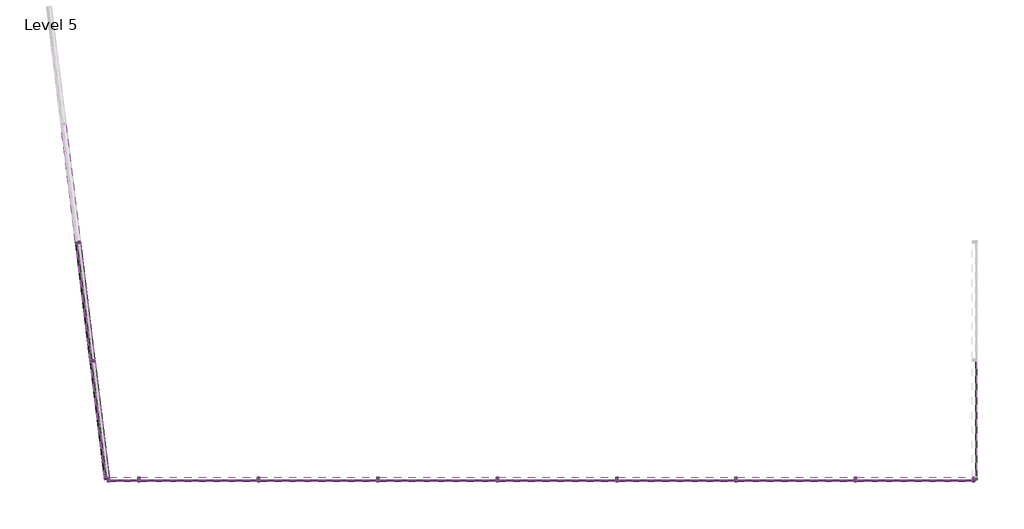
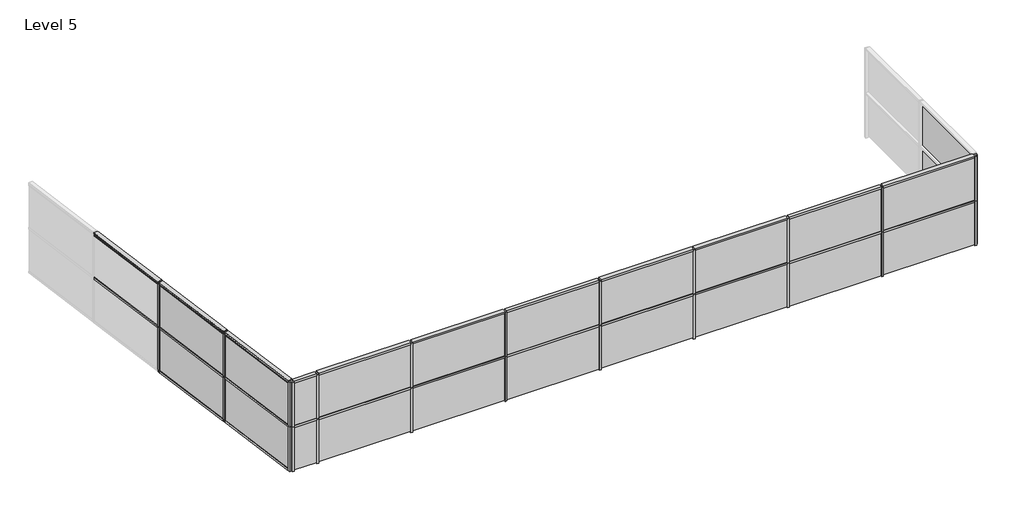
# One storey, part 1 of 2: 62 members, 26 plates.
"""IFC4 building model written with IfcOpenShell, lengths in millimetres."""

from ifc_helpers import new_model, si_unit, origin, place, context, project, spatial, transform, mapped, element, save
from components import member_71c27fd2, member_daa7a266, member_82905deb, member_19d0a4ec, member_8cef0660, member_db480205, member_4491d118, member_0c11e56c, system_panel_glazed_37f15d2e, system_panel_glazed_3620f98e, system_panel_glazed_e46d4b42, system_panel_glazed_2a6c68b7, system_panel_glazed_9d0e0944

model = new_model("IFC4")

# Units and contexts
model_context = context("Model", 3, world=origin())
ifc_project = project(units=[si_unit("LENGTHUNIT", "METRE", prefix="MILLI")], contexts=[model_context])

# Site, building, storey
site = spatial("IfcSite", under=ifc_project)
building = spatial("IfcBuilding", under=site)
storey = spatial("IfcBuildingStorey", under=building, Name="Level 5", Elevation=12192.0)

# Members
placement = place(None, origin())
member_shape = member_71c27fd2(model_context)
element("IfcMember", 1, ObjectType="Rectangular Mullion : 2.5\" x 5\" rectangular", at=placement, inside=storey, context=model_context, shape_type="MappedRepresentation", body=[
    mapped(member_shape, transform((-8620.3262186, -3985.3690403, 12192.0), x_axis=(0.0, 0.0, -1.0), y_axis=(-0.9925461516413222, -0.12186934340514607, 0.0), z_axis=(-0.12186934340514607, 0.9925461516413222, 0.0))),
])
member_2_shape = member_daa7a266(model_context)
element("IfcMember", 2, ObjectType="Rectangular Mullion : 2.5\" x 5\" rectangular", at=placement, inside=storey, context=model_context, shape_type="MappedRepresentation", body=[
    mapped(member_2_shape, transform((-8260.4765148, -6916.1096898, 15240.0), x_axis=(0.0, 0.0, 1.0), y_axis=(-0.9925461516413222, -0.12186934340514587, 0.0), z_axis=(0.12186934340514587, -0.9925461516413222, 0.0))),
])
member_3_shape = member_82905deb(model_context)
element("IfcMember", 3, ObjectType="Rectangular Mullion : 2.5\" x 5\" rectangular", at=placement, inside=storey, context=model_context, shape_type="MappedRepresentation", body=[
    mapped(member_3_shape, transform((-8624.1955702, -3953.8557, 15240.0), x_axis=(-0.1218693434051459, 0.9925461516413222, 0.0), y_axis=(-0.9925461516413222, -0.1218693434051459, 0.0), z_axis=(0.0, 0.0, 1.0))),
])
element("IfcMember", 4, ObjectType="Rectangular Mullion : 2.5\" x 5\" rectangular", at=placement, inside=storey, context=model_context, shape_type="MappedRepresentation", body=[
    mapped(member_3_shape, transform((-8995.6533289, -928.5750297, 15240.0), x_axis=(-0.1218693434051459, 0.9925461516413222, 0.0), y_axis=(-0.9925461516413222, -0.1218693434051459, 0.0), z_axis=(0.0, 0.0, 1.0))),
])
member_4_shape = member_19d0a4ec(model_context)
element("IfcMember", 5, ObjectType="Rectangular Mullion : 2.5\" x 5\" rectangular", at=placement, inside=storey, context=model_context, shape_type="MappedRepresentation", body=[
    mapped(member_4_shape, transform((13839.0156363, -6979.1363705, 13716.0), x_axis=(0.0, 0.0, 1.0), y_axis=(0.0, -1.0, 0.0), z_axis=(1.0, 0.0, 0.0))),
])
element("IfcMember", 6, ObjectType="Rectangular Mullion : 2.5\" x 5\" rectangular", at=placement, inside=storey, context=model_context, shape_type="MappedRepresentation", body=[
    mapped(member_4_shape, transform((13839.0156363, -6979.1363705, 15240.0), x_axis=(0.0, 0.0, 1.0), y_axis=(0.0, -1.0, 0.0), z_axis=(1.0, 0.0, 0.0))),
])
element("IfcMember", 7, ObjectType="Rectangular Mullion : 2.5\" x 5\" rectangular", at=placement, inside=storey, context=model_context, shape_type="MappedRepresentation", body=[
    mapped(member_4_shape, transform((-8260.4765148, -6916.1096898, 13716.0), x_axis=(0.0, 0.0, 1.0), y_axis=(-0.9925461516413222, -0.12186934340514591, 0.0), z_axis=(0.12186934340514591, -0.9925461516413222, 0.0))),
])
element("IfcMember", 8, ObjectType="Rectangular Mullion : 2.5\" x 5\" rectangular", at=placement, inside=storey, context=model_context, shape_type="MappedRepresentation", body=[
    mapped(member_4_shape, transform((-8260.4765148, -6916.1096898, 15240.0), x_axis=(0.0, 0.0, 1.0), y_axis=(-0.9925461516413223, -0.12186934340514578, 0.0), z_axis=(0.12186934340514578, -0.9925461516413223, 0.0))),
])
element("IfcMember", 9, ObjectType="Rectangular Mullion : 2.5\" x 5\" rectangular", at=placement, inside=storey, context=model_context, shape_type="MappedRepresentation", body=[
    mapped(member_4_shape, transform((-8260.4765148, -6916.1096898, 13716.0), x_axis=(0.0, 0.0, 1.0), y_axis=(-0.9925461516413223, -0.1218693434051456, 0.0), z_axis=(0.12186934340514559, -0.9925461516413222, 0.0))),
])
member_5_shape = member_8cef0660(model_context)
element("IfcMember", 10, ObjectType="Rectangular Mullion : 2.5\" x 5\" rectangular", at=placement, inside=storey, context=model_context, shape_type="MappedRepresentation", body=[
    mapped(member_5_shape, transform((10822.765636, -6979.1363705, 13716.0), x_axis=(0.0, 0.0, 1.0), y_axis=(0.0, -1.0, 0.0), z_axis=(1.0, 0.0, 0.0))),
])
element("IfcMember", 11, ObjectType="Rectangular Mullion : 2.5\" x 5\" rectangular", at=placement, inside=storey, context=model_context, shape_type="MappedRepresentation", body=[
    mapped(member_5_shape, transform((7774.765636, -6979.1363705, 13716.0), x_axis=(0.0, 0.0, 1.0), y_axis=(0.0, -1.0, 0.0), z_axis=(1.0, 0.0, 0.0))),
])
element("IfcMember", 12, ObjectType="Rectangular Mullion : 2.5\" x 5\" rectangular", at=placement, inside=storey, context=model_context, shape_type="MappedRepresentation", body=[
    mapped(member_5_shape, transform((4726.765636, -6979.1363705, 13716.0), x_axis=(0.0, 0.0, 1.0), y_axis=(0.0, -1.0, 0.0), z_axis=(1.0, 0.0, 0.0))),
])
element("IfcMember", 13, ObjectType="Rectangular Mullion : 2.5\" x 5\" rectangular", at=placement, inside=storey, context=model_context, shape_type="MappedRepresentation", body=[
    mapped(member_5_shape, transform((1678.765636, -6979.1363705, 13716.0), x_axis=(0.0, 0.0, 1.0), y_axis=(0.0, -1.0, 0.0), z_axis=(1.0, 0.0, 0.0))),
])
element("IfcMember", 14, ObjectType="Rectangular Mullion : 2.5\" x 5\" rectangular", at=placement, inside=storey, context=model_context, shape_type="MappedRepresentation", body=[
    mapped(member_5_shape, transform((-1369.234364, -6979.1363705, 13716.0), x_axis=(0.0, 0.0, 1.0), y_axis=(0.0, -1.0, 0.0), z_axis=(1.0, 0.0, 0.0))),
])
element("IfcMember", 15, ObjectType="Rectangular Mullion : 2.5\" x 5\" rectangular", at=placement, inside=storey, context=model_context, shape_type="MappedRepresentation", body=[
    mapped(member_5_shape, transform((-4417.234364, -6979.1363705, 13716.0), x_axis=(0.0, 0.0, 1.0), y_axis=(0.0, -1.0, 0.0), z_axis=(1.0, 0.0, 0.0))),
])
element("IfcMember", 16, ObjectType="Rectangular Mullion : 2.5\" x 5\" rectangular", at=placement, inside=storey, context=model_context, shape_type="MappedRepresentation", body=[
    mapped(member_5_shape, transform((10822.765636, -6979.1363705, 15240.0), x_axis=(0.0, 0.0, 1.0), y_axis=(0.0, -1.0, 0.0), z_axis=(1.0, 0.0, 0.0))),
])
element("IfcMember", 17, ObjectType="Rectangular Mullion : 2.5\" x 5\" rectangular", at=placement, inside=storey, context=model_context, shape_type="MappedRepresentation", body=[
    mapped(member_5_shape, transform((7774.765636, -6979.1363705, 15240.0), x_axis=(0.0, 0.0, 1.0), y_axis=(0.0, -1.0, 0.0), z_axis=(1.0, 0.0, 0.0))),
])
element("IfcMember", 18, ObjectType="Rectangular Mullion : 2.5\" x 5\" rectangular", at=placement, inside=storey, context=model_context, shape_type="MappedRepresentation", body=[
    mapped(member_5_shape, transform((4726.765636, -6979.1363705, 15240.0), x_axis=(0.0, 0.0, 1.0), y_axis=(0.0, -1.0, 0.0), z_axis=(1.0, 0.0, 0.0))),
])
element("IfcMember", 19, ObjectType="Rectangular Mullion : 2.5\" x 5\" rectangular", at=placement, inside=storey, context=model_context, shape_type="MappedRepresentation", body=[
    mapped(member_5_shape, transform((1678.765636, -6979.1363705, 15240.0), x_axis=(0.0, 0.0, 1.0), y_axis=(0.0, -1.0, 0.0), z_axis=(1.0, 0.0, 0.0))),
])
element("IfcMember", 20, ObjectType="Rectangular Mullion : 2.5\" x 5\" rectangular", at=placement, inside=storey, context=model_context, shape_type="MappedRepresentation", body=[
    mapped(member_5_shape, transform((-1369.234364, -6979.1363705, 15240.0), x_axis=(0.0, 0.0, 1.0), y_axis=(0.0, -1.0, 0.0), z_axis=(1.0, 0.0, 0.0))),
])
element("IfcMember", 21, ObjectType="Rectangular Mullion : 2.5\" x 5\" rectangular", at=placement, inside=storey, context=model_context, shape_type="MappedRepresentation", body=[
    mapped(member_5_shape, transform((-4417.234364, -6979.1363705, 15240.0), x_axis=(0.0, 0.0, 1.0), y_axis=(0.0, -1.0, 0.0), z_axis=(1.0, 0.0, 0.0))),
])
element("IfcMember", 22, ObjectType="Rectangular Mullion : 2.5\" x 5\" rectangular", at=placement, inside=storey, context=model_context, shape_type="MappedRepresentation", body=[
    mapped(member_5_shape, transform((-8628.0649219, -3922.3423596, 13716.0), x_axis=(0.0, 0.0, 1.0), y_axis=(-0.9925461516413222, -0.12186934340514592, 0.0), z_axis=(0.12186934340514592, -0.9925461516413222, 0.0))),
])
element("IfcMember", 23, ObjectType="Rectangular Mullion : 2.5\" x 5\" rectangular", at=placement, inside=storey, context=model_context, shape_type="MappedRepresentation", body=[
    mapped(member_5_shape, transform((-8999.5226806, -897.0616894, 13716.0), x_axis=(0.0, 0.0, 1.0), y_axis=(-0.9925461516413222, -0.12186934340514566, 0.0), z_axis=(0.12186934340514566, -0.9925461516413222, 0.0))),
])
element("IfcMember", 24, ObjectType="Rectangular Mullion : 2.5\" x 5\" rectangular", at=placement, inside=storey, context=model_context, shape_type="MappedRepresentation", body=[
    mapped(member_5_shape, transform((-8628.0649219, -3922.3423596, 15240.0), x_axis=(0.0, 0.0, 1.0), y_axis=(-0.9925461516413222, -0.12186934340514592, 0.0), z_axis=(0.12186934340514592, -0.9925461516413222, 0.0))),
])
element("IfcMember", 25, ObjectType="Rectangular Mullion : 2.5\" x 5\" rectangular", at=placement, inside=storey, context=model_context, shape_type="MappedRepresentation", body=[
    mapped(member_5_shape, transform((-8999.5226806, -897.0616894, 15240.0), x_axis=(0.0, 0.0, 1.0), y_axis=(-0.9925461516413222, -0.12186934340514602, 0.0), z_axis=(0.12186934340514602, -0.9925461516413222, 0.0))),
])
element("IfcMember", 26, ObjectType="Rectangular Mullion : 2.5\" x 5\" rectangular", at=placement, inside=storey, context=model_context, shape_type="MappedRepresentation", body=[
    mapped(member_5_shape, transform((-8628.0649219, -3922.3423596, 13716.0), x_axis=(0.0, 0.0, 1.0), y_axis=(-0.9925461516413222, -0.12186934340514595, 0.0), z_axis=(0.12186934340514595, -0.9925461516413222, 0.0))),
])
element("IfcMember", 27, ObjectType="Rectangular Mullion : 2.5\" x 5\" rectangular", at=placement, inside=storey, context=model_context, shape_type="MappedRepresentation", body=[
    mapped(member_5_shape, transform((-8999.5226806, -897.0616894, 13716.0), x_axis=(0.0, 0.0, 1.0), y_axis=(-0.9925461516413222, -0.12186934340514599, 0.0), z_axis=(0.12186934340514599, -0.9925461516413222, 0.0))),
])
member_6_shape = member_db480205(model_context)
element("IfcMember", 28, ObjectType="Rectangular Mullion : 2.5\" x 5\" rectangular", at=placement, inside=storey, context=model_context, shape_type="MappedRepresentation", body=[
    mapped(member_6_shape, transform((-8991.7839773, -960.0883701, 12192.0), x_axis=(0.0, 0.0, -1.0), y_axis=(-0.9925461516413222, -0.12186934340514592, 0.0), z_axis=(-0.12186934340514592, 0.9925461516413222, 0.0))),
])
element("IfcMember", 29, ObjectType="Rectangular Mullion : 2.5\" x 5\" rectangular", at=placement, inside=storey, context=model_context, shape_type="MappedRepresentation", body=[
    mapped(member_6_shape, transform((-8628.0649219, -3922.3423596, 15240.0), x_axis=(0.0, 0.0, 1.0), y_axis=(-0.9925461516413222, -0.12186934340514592, 0.0), z_axis=(0.12186934340514592, -0.9925461516413222, 0.0))),
])
element("IfcMember", 30, ObjectType="Rectangular Mullion : 2.5\" x 5\" rectangular", at=placement, inside=storey, context=model_context, shape_type="MappedRepresentation", body=[
    mapped(member_6_shape, transform((-8999.5226806, -897.0616894, 15240.0), x_axis=(0.0, 0.0, 1.0), y_axis=(-0.9925461516413222, -0.12186934340514596, 0.0), z_axis=(0.12186934340514596, -0.9925461516413222, 0.0))),
])
element("IfcMember", 31, ObjectType="Rectangular Mullion : 2.5\" x 5\" rectangular", at=placement, inside=storey, context=model_context, shape_type="MappedRepresentation", body=[
    mapped(member_3_shape, transform((-8624.1955702, -3953.8557, 13716.0), x_axis=(-0.1218693434051459, 0.9925461516413222, 0.0), y_axis=(-0.9925461516413222, -0.1218693434051459, 0.0), z_axis=(0.0, 0.0, 1.0))),
])
element("IfcMember", 32, ObjectType="Rectangular Mullion : 2.5\" x 5\" rectangular", at=placement, inside=storey, context=model_context, shape_type="MappedRepresentation", body=[
    mapped(member_3_shape, transform((-8995.6533289, -928.5750297, 13716.0), x_axis=(-0.1218693434051459, 0.9925461516413222, 0.0), y_axis=(-0.9925461516413222, -0.1218693434051459, 0.0), z_axis=(0.0, 0.0, 1.0))),
])
element("IfcMember", 33, ObjectType="Rectangular Mullion : 2.5\" x 5\" rectangular", at=placement, inside=storey, context=model_context, shape_type="MappedRepresentation", body=[
    mapped(member_3_shape, transform((10854.515636, -6979.1363705, 13716.0), x_axis=(-1.0, 0.0, 0.0), y_axis=(0.0, -1.0, 0.0), z_axis=(0.0, 0.0, 1.0))),
])
element("IfcMember", 34, ObjectType="Rectangular Mullion : 2.5\" x 5\" rectangular", at=placement, inside=storey, context=model_context, shape_type="MappedRepresentation", body=[
    mapped(member_3_shape, transform((10854.515636, -6979.1363705, 15240.0), x_axis=(-1.0, 0.0, 0.0), y_axis=(0.0, -1.0, 0.0), z_axis=(0.0, 0.0, 1.0))),
])
element("IfcMember", 35, ObjectType="Rectangular Mullion : 2.5\" x 5\" rectangular", at=placement, inside=storey, context=model_context, shape_type="MappedRepresentation", body=[
    mapped(member_3_shape, transform((7806.515636, -6979.1363705, 13716.0), x_axis=(-1.0, 0.0, 0.0), y_axis=(0.0, -1.0, 0.0), z_axis=(0.0, 0.0, 1.0))),
])
element("IfcMember", 36, ObjectType="Rectangular Mullion : 2.5\" x 5\" rectangular", at=placement, inside=storey, context=model_context, shape_type="MappedRepresentation", body=[
    mapped(member_3_shape, transform((7806.515636, -6979.1363705, 15240.0), x_axis=(-1.0, 0.0, 0.0), y_axis=(0.0, -1.0, 0.0), z_axis=(0.0, 0.0, 1.0))),
])
element("IfcMember", 37, ObjectType="Rectangular Mullion : 2.5\" x 5\" rectangular", at=placement, inside=storey, context=model_context, shape_type="MappedRepresentation", body=[
    mapped(member_3_shape, transform((4758.515636, -6979.1363705, 13716.0), x_axis=(-1.0, 0.0, 0.0), y_axis=(0.0, -1.0, 0.0), z_axis=(0.0, 0.0, 1.0))),
])
element("IfcMember", 38, ObjectType="Rectangular Mullion : 2.5\" x 5\" rectangular", at=placement, inside=storey, context=model_context, shape_type="MappedRepresentation", body=[
    mapped(member_3_shape, transform((4758.515636, -6979.1363705, 15240.0), x_axis=(-1.0, 0.0, 0.0), y_axis=(0.0, -1.0, 0.0), z_axis=(0.0, 0.0, 1.0))),
])
element("IfcMember", 39, ObjectType="Rectangular Mullion : 2.5\" x 5\" rectangular", at=placement, inside=storey, context=model_context, shape_type="MappedRepresentation", body=[
    mapped(member_3_shape, transform((1710.515636, -6979.1363705, 13716.0), x_axis=(-1.0, 0.0, 0.0), y_axis=(0.0, -1.0, 0.0), z_axis=(0.0, 0.0, 1.0))),
])
element("IfcMember", 40, ObjectType="Rectangular Mullion : 2.5\" x 5\" rectangular", at=placement, inside=storey, context=model_context, shape_type="MappedRepresentation", body=[
    mapped(member_3_shape, transform((1710.515636, -6979.1363705, 15240.0), x_axis=(-1.0, 0.0, 0.0), y_axis=(0.0, -1.0, 0.0), z_axis=(0.0, 0.0, 1.0))),
])
element("IfcMember", 41, ObjectType="Rectangular Mullion : 2.5\" x 5\" rectangular", at=placement, inside=storey, context=model_context, shape_type="MappedRepresentation", body=[
    mapped(member_3_shape, transform((-1337.484364, -6979.1363705, 13716.0), x_axis=(-1.0, 0.0, 0.0), y_axis=(0.0, -1.0, 0.0), z_axis=(0.0, 0.0, 1.0))),
])
element("IfcMember", 42, ObjectType="Rectangular Mullion : 2.5\" x 5\" rectangular", at=placement, inside=storey, context=model_context, shape_type="MappedRepresentation", body=[
    mapped(member_3_shape, transform((-1337.484364, -6979.1363705, 15240.0), x_axis=(-1.0, 0.0, 0.0), y_axis=(0.0, -1.0, 0.0), z_axis=(0.0, 0.0, 1.0))),
])
element("IfcMember", 43, ObjectType="Rectangular Mullion : 2.5\" x 5\" rectangular", at=placement, inside=storey, context=model_context, shape_type="MappedRepresentation", body=[
    mapped(member_3_shape, transform((-4385.484364, -6979.1363705, 13716.0), x_axis=(-1.0, 0.0, 0.0), y_axis=(0.0, -1.0, 0.0), z_axis=(0.0, 0.0, 1.0))),
])
element("IfcMember", 44, ObjectType="Rectangular Mullion : 2.5\" x 5\" rectangular", at=placement, inside=storey, context=model_context, shape_type="MappedRepresentation", body=[
    mapped(member_3_shape, transform((-4385.484364, -6979.1363705, 15240.0), x_axis=(-1.0, 0.0, 0.0), y_axis=(0.0, -1.0, 0.0), z_axis=(0.0, 0.0, 1.0))),
])
element("IfcMember", 45, ObjectType="Rectangular Mullion : 2.5\" x 5\" rectangular", at=placement, inside=storey, context=model_context, shape_type="MappedRepresentation", body=[
    mapped(member_3_shape, transform((-7433.484364, -6979.1363705, 13716.0), x_axis=(-1.0, 0.0, 0.0), y_axis=(0.0, -1.0, 0.0), z_axis=(0.0, 0.0, 1.0))),
])
element("IfcMember", 46, ObjectType="Rectangular Mullion : 2.5\" x 5\" rectangular", at=placement, inside=storey, context=model_context, shape_type="MappedRepresentation", body=[
    mapped(member_3_shape, transform((-7433.484364, -6979.1363705, 15240.0), x_axis=(-1.0, 0.0, 0.0), y_axis=(0.0, -1.0, 0.0), z_axis=(0.0, 0.0, 1.0))),
])
element("IfcMember", 47, ObjectType="Rectangular Mullion : 2.5\" x 5\" rectangular", at=placement, inside=storey, context=model_context, shape_type="MappedRepresentation", body=[
    mapped(member_3_shape, transform((-8624.1955702, -3953.8557, 15240.0), x_axis=(-0.1218693434051459, 0.9925461516413222, 0.0), y_axis=(-0.9925461516413222, -0.1218693434051459, 0.0), z_axis=(0.0, 0.0, 1.0))),
])
element("IfcMember", 48, ObjectType="Rectangular Mullion : 2.5\" x 5\" rectangular", at=placement, inside=storey, context=model_context, shape_type="MappedRepresentation", body=[
    mapped(member_3_shape, transform((-8995.6533289, -928.5750297, 15240.0), x_axis=(-0.1218693434051459, 0.9925461516413222, 0.0), y_axis=(-0.9925461516413222, -0.1218693434051459, 0.0), z_axis=(0.0, 0.0, 1.0))),
])
element("IfcMember", 49, ObjectType="Rectangular Mullion : 2.5\" x 5\" rectangular", at=placement, inside=storey, context=model_context, shape_type="MappedRepresentation", body=[
    mapped(member_3_shape, transform((-8624.1955702, -3953.8557, 13716.0), x_axis=(-0.1218693434051459, 0.9925461516413222, 0.0), y_axis=(-0.9925461516413222, -0.1218693434051459, 0.0), z_axis=(0.0, 0.0, 1.0))),
])
element("IfcMember", 50, ObjectType="Rectangular Mullion : 2.5\" x 5\" rectangular", at=placement, inside=storey, context=model_context, shape_type="MappedRepresentation", body=[
    mapped(member_3_shape, transform((-8995.6533289, -928.5750297, 13716.0), x_axis=(-0.1218693434051459, 0.9925461516413222, 0.0), y_axis=(-0.9925461516413222, -0.1218693434051459, 0.0), z_axis=(0.0, 0.0, 1.0))),
])
member_7_shape = member_4491d118(model_context)
element("IfcMember", 51, ObjectType="Rectangular Mullion : 2.5\" x 5\" rectangular", at=placement, inside=storey, context=model_context, shape_type="MappedRepresentation", body=[
    mapped(member_7_shape, transform((-8252.7378115, -6979.1363705, 12192.0), x_axis=(0.1218693434051459, -0.9925461516413222, 0.0), y_axis=(-0.9925461516413222, -0.1218693434051459, 0.0), z_axis=(0.0, 0.0, -1.0))),
])
element("IfcMember", 52, ObjectType="Rectangular Mullion : 2.5\" x 5\" rectangular", at=placement, inside=storey, context=model_context, shape_type="MappedRepresentation", body=[
    mapped(member_7_shape, transform((13902.5156363, -6979.1363705, 12192.0), x_axis=(1.0, 0.0, 0.0), y_axis=(0.0, -1.0, 0.0), z_axis=(0.0, 0.0, -1.0))),
])
element("IfcMember", 53, ObjectType="Rectangular Mullion : 2.5\" x 5\" rectangular", at=placement, inside=storey, context=model_context, shape_type="MappedRepresentation", body=[
    mapped(member_7_shape, transform((13902.5156363, -6979.1363705, 13716.0), x_axis=(1.0, 0.0, 0.0), y_axis=(0.0, -1.0, 0.0), z_axis=(0.0, 0.0, -1.0))),
])
element("IfcMember", 54, ObjectType="Rectangular Mullion : 2.5\" x 5\" rectangular", at=placement, inside=storey, context=model_context, shape_type="MappedRepresentation", body=[
    mapped(member_7_shape, transform((-8252.7378115, -6979.1363705, 13716.0), x_axis=(0.1218693434051459, -0.9925461516413222, 0.0), y_axis=(-0.9925461516413222, -0.1218693434051459, 0.0), z_axis=(0.0, 0.0, -1.0))),
])
element("IfcMember", 55, ObjectType="Rectangular Mullion : 2.5\" x 5\" rectangular", at=placement, inside=storey, context=model_context, shape_type="MappedRepresentation", body=[
    mapped(member_7_shape, transform((-8252.7378115, -6979.1363705, 12192.0), x_axis=(0.1218693434051459, -0.9925461516413222, 0.0), y_axis=(-0.9925461516413222, -0.1218693434051459, 0.0), z_axis=(0.0, 0.0, -1.0))),
])
element("IfcMember", 56, ObjectType="Rectangular Mullion : 2.5\" x 5\" rectangular", at=placement, inside=storey, context=model_context, shape_type="MappedRepresentation", body=[
    mapped(member_7_shape, transform((-8252.7378115, -6979.1363705, 13716.0), x_axis=(0.1218693434051459, -0.9925461516413222, 0.0), y_axis=(-0.9925461516413222, -0.1218693434051459, 0.0), z_axis=(0.0, 0.0, -1.0))),
])
element("IfcMember", 57, ObjectType="Rectangular Mullion : 2.5\" x 5\" rectangular", at=placement, inside=storey, context=model_context, shape_type="MappedRepresentation", body=[
    mapped(member_7_shape, transform((-8252.7378115, -6979.1363705, 13716.0), x_axis=(-1.0, 0.0, 0.0), y_axis=(0.0, -1.0, 0.0), z_axis=(0.0, 0.0, 1.0))),
])
element("IfcMember", 58, ObjectType="Rectangular Mullion : 2.5\" x 5\" rectangular", at=placement, inside=storey, context=model_context, shape_type="MappedRepresentation", body=[
    mapped(member_7_shape, transform((-8252.7378115, -6979.1363705, 15240.0), x_axis=(-1.0, 0.0, 0.0), y_axis=(0.0, -1.0, 0.0), z_axis=(0.0, 0.0, 1.0))),
])
element("IfcMember", 59, ObjectType="Rectangular Mullion : 2.5\" x 5\" rectangular", at=placement, inside=storey, context=model_context, shape_type="MappedRepresentation", body=[
    mapped(member_7_shape, transform((13902.5156363, -6979.1363705, 13716.0), x_axis=(0.0, -1.0, 0.0), y_axis=(1.0, 0.0, 0.0), z_axis=(0.0, 0.0, 1.0))),
])
element("IfcMember", 60, ObjectType="Rectangular Mullion : 2.5\" x 5\" rectangular", at=placement, inside=storey, context=model_context, shape_type="MappedRepresentation", body=[
    mapped(member_7_shape, transform((13902.5156363, -6979.1363705, 15240.0), x_axis=(0.0, -1.0, 0.0), y_axis=(1.0, 0.0, 0.0), z_axis=(0.0, 0.0, 1.0))),
])
member_8_shape = member_0c11e56c(model_context)
element("IfcMember", 61, ObjectType="Rectangular Mullion : 2.5\" x 5\" rectangular", at=placement, inside=storey, context=model_context, shape_type="MappedRepresentation", body=[
    mapped(member_8_shape, transform((-7465.234364, -6979.1363705, 13716.0), x_axis=(0.0, 0.0, 1.0), y_axis=(0.0, -1.0, 0.0), z_axis=(1.0, 0.0, 0.0))),
])
element("IfcMember", 62, ObjectType="Rectangular Mullion : 2.5\" x 5\" rectangular", at=placement, inside=storey, context=model_context, shape_type="MappedRepresentation", body=[
    mapped(member_8_shape, transform((-7465.234364, -6979.1363705, 15240.0), x_axis=(0.0, 0.0, 1.0), y_axis=(0.0, -1.0, 0.0), z_axis=(1.0, 0.0, 0.0))),
])

# Plates
system_panel_glazed_shape = system_panel_glazed_37f15d2e(model_context)
element("IfcPlate", 63, ObjectType="System Panel : Glazed", at=placement, inside=storey, context=model_context, shape_type="MappedRepresentation", body=[
    mapped(system_panel_glazed_shape, transform((-8440.4013667, -5450.739365, 12255.5), x_axis=(-0.1218693434051459, 0.9925461516413222, 0.0), y_axis=(-0.9925461516413222, -0.1218693434051459, 0.0), z_axis=(0.0, 0.0, 1.0))),
])
element("IfcPlate", 64, ObjectType="System Panel : Glazed", at=placement, inside=storey, context=model_context, shape_type="MappedRepresentation", body=[
    mapped(system_panel_glazed_shape, transform((-8440.4013667, -5450.739365, 13747.75), x_axis=(-0.1218693434051459, 0.9925461516413222, 0.0), y_axis=(-0.9925461516413222, -0.1218693434051459, 0.0), z_axis=(0.0, 0.0, 1.0))),
])
system_panel_glazed_2_shape = system_panel_glazed_3620f98e(model_context)
element("IfcPlate", 65, ObjectType="System Panel : Glazed", at=placement, inside=storey, context=model_context, shape_type="MappedRepresentation", body=[
    mapped(system_panel_glazed_2_shape, transform((-8809.9244496, -2441.2153649, 13747.75), x_axis=(-0.1218693434051459, 0.9925461516413222, 0.0), y_axis=(-0.9925461516413222, -0.1218693434051459, 0.0), z_axis=(0.0, 0.0, 1.0))),
])
element("IfcPlate", 66, ObjectType="System Panel : Glazed", at=placement, inside=storey, context=model_context, shape_type="MappedRepresentation", body=[
    mapped(system_panel_glazed_2_shape, transform((-8809.9244496, -2441.2153649, 12255.5), x_axis=(-0.1218693434051459, 0.9925461516413222, 0.0), y_axis=(-0.9925461516413222, -0.1218693434051459, 0.0), z_axis=(0.0, 0.0, 1.0))),
])
system_panel_glazed_3_shape = system_panel_glazed_e46d4b42(model_context)
element("IfcPlate", 67, ObjectType="System Panel : Glazed", at=placement, inside=storey, context=model_context, shape_type="MappedRepresentation", body=[
    mapped(system_panel_glazed_3_shape, transform((-8440.4013667, -5450.739365, 12223.75), x_axis=(-0.1218693434051459, 0.9925461516413222, 0.0), y_axis=(-0.9925461516413222, -0.1218693434051459, 0.0), z_axis=(0.0, 0.0, 1.0))),
])
element("IfcPlate", 68, ObjectType="System Panel : Glazed", at=placement, inside=storey, context=model_context, shape_type="MappedRepresentation", body=[
    mapped(system_panel_glazed_3_shape, transform((12362.6406361, -6979.1363705, 12223.75), x_axis=(-1.0, 0.0, 0.0), y_axis=(0.0, -1.0, 0.0), z_axis=(0.0, 0.0, 1.0))),
])
element("IfcPlate", 69, ObjectType="System Panel : Glazed", at=placement, inside=storey, context=model_context, shape_type="MappedRepresentation", body=[
    mapped(system_panel_glazed_3_shape, transform((12362.6406361, -6979.1363705, 13747.75), x_axis=(-1.0, 0.0, 0.0), y_axis=(0.0, -1.0, 0.0), z_axis=(0.0, 0.0, 1.0))),
])
element("IfcPlate", 70, ObjectType="System Panel : Glazed", at=placement, inside=storey, context=model_context, shape_type="MappedRepresentation", body=[
    mapped(system_panel_glazed_3_shape, transform((13902.5156363, -5439.2613706, 12223.75), x_axis=(0.0, -1.0, 0.0), y_axis=(1.0, 0.0, 0.0), z_axis=(0.0, 0.0, 1.0))),
])
element("IfcPlate", 71, ObjectType="System Panel : Glazed", at=placement, inside=storey, context=model_context, shape_type="MappedRepresentation", body=[
    mapped(system_panel_glazed_3_shape, transform((13902.5156363, -5439.2613706, 13747.75), x_axis=(0.0, -1.0, 0.0), y_axis=(1.0, 0.0, 0.0), z_axis=(0.0, 0.0, 1.0))),
])
element("IfcPlate", 72, ObjectType="System Panel : Glazed", at=placement, inside=storey, context=model_context, shape_type="MappedRepresentation", body=[
    mapped(system_panel_glazed_3_shape, transform((-8440.4013667, -5450.739365, 13747.75), x_axis=(-0.1218693434051459, 0.9925461516413222, 0.0), y_axis=(-0.9925461516413222, -0.1218693434051459, 0.0), z_axis=(0.0, 0.0, 1.0))),
])
system_panel_glazed_4_shape = system_panel_glazed_2a6c68b7(model_context)
element("IfcPlate", 73, ObjectType="System Panel : Glazed", at=placement, inside=storey, context=model_context, shape_type="MappedRepresentation", body=[
    mapped(system_panel_glazed_4_shape, transform((-8809.9244496, -2441.2153649, 12223.75), x_axis=(-0.1218693434051459, 0.9925461516413222, 0.0), y_axis=(-0.9925461516413222, -0.1218693434051459, 0.0), z_axis=(0.0, 0.0, 1.0))),
])
element("IfcPlate", 74, ObjectType="System Panel : Glazed", at=placement, inside=storey, context=model_context, shape_type="MappedRepresentation", body=[
    mapped(system_panel_glazed_4_shape, transform((9330.515636, -6979.1363705, 12223.75), x_axis=(-1.0, 0.0, 0.0), y_axis=(0.0, -1.0, 0.0), z_axis=(0.0, 0.0, 1.0))),
])
element("IfcPlate", 75, ObjectType="System Panel : Glazed", at=placement, inside=storey, context=model_context, shape_type="MappedRepresentation", body=[
    mapped(system_panel_glazed_4_shape, transform((6282.515636, -6979.1363705, 12223.75), x_axis=(-1.0, 0.0, 0.0), y_axis=(0.0, -1.0, 0.0), z_axis=(0.0, 0.0, 1.0))),
])
element("IfcPlate", 76, ObjectType="System Panel : Glazed", at=placement, inside=storey, context=model_context, shape_type="MappedRepresentation", body=[
    mapped(system_panel_glazed_4_shape, transform((3234.515636, -6979.1363705, 12223.75), x_axis=(-1.0, 0.0, 0.0), y_axis=(0.0, -1.0, 0.0), z_axis=(0.0, 0.0, 1.0))),
])
element("IfcPlate", 77, ObjectType="System Panel : Glazed", at=placement, inside=storey, context=model_context, shape_type="MappedRepresentation", body=[
    mapped(system_panel_glazed_4_shape, transform((186.515636, -6979.1363705, 12223.75), x_axis=(-1.0, 0.0, 0.0), y_axis=(0.0, -1.0, 0.0), z_axis=(0.0, 0.0, 1.0))),
])
element("IfcPlate", 78, ObjectType="System Panel : Glazed", at=placement, inside=storey, context=model_context, shape_type="MappedRepresentation", body=[
    mapped(system_panel_glazed_4_shape, transform((-2861.484364, -6979.1363705, 12223.75), x_axis=(-1.0, 0.0, 0.0), y_axis=(0.0, -1.0, 0.0), z_axis=(0.0, 0.0, 1.0))),
])
element("IfcPlate", 79, ObjectType="System Panel : Glazed", at=placement, inside=storey, context=model_context, shape_type="MappedRepresentation", body=[
    mapped(system_panel_glazed_4_shape, transform((-5909.484364, -6979.1363705, 12223.75), x_axis=(-1.0, 0.0, 0.0), y_axis=(0.0, -1.0, 0.0), z_axis=(0.0, 0.0, 1.0))),
])
element("IfcPlate", 80, ObjectType="System Panel : Glazed", at=placement, inside=storey, context=model_context, shape_type="MappedRepresentation", body=[
    mapped(system_panel_glazed_4_shape, transform((9330.515636, -6979.1363705, 13747.75), x_axis=(-1.0, 0.0, 0.0), y_axis=(0.0, -1.0, 0.0), z_axis=(0.0, 0.0, 1.0))),
])
element("IfcPlate", 81, ObjectType="System Panel : Glazed", at=placement, inside=storey, context=model_context, shape_type="MappedRepresentation", body=[
    mapped(system_panel_glazed_4_shape, transform((6282.515636, -6979.1363705, 13747.75), x_axis=(-1.0, 0.0, 0.0), y_axis=(0.0, -1.0, 0.0), z_axis=(0.0, 0.0, 1.0))),
])
element("IfcPlate", 82, ObjectType="System Panel : Glazed", at=placement, inside=storey, context=model_context, shape_type="MappedRepresentation", body=[
    mapped(system_panel_glazed_4_shape, transform((3234.515636, -6979.1363705, 13747.75), x_axis=(-1.0, 0.0, 0.0), y_axis=(0.0, -1.0, 0.0), z_axis=(0.0, 0.0, 1.0))),
])
element("IfcPlate", 83, ObjectType="System Panel : Glazed", at=placement, inside=storey, context=model_context, shape_type="MappedRepresentation", body=[
    mapped(system_panel_glazed_4_shape, transform((186.515636, -6979.1363705, 13747.75), x_axis=(-1.0, 0.0, 0.0), y_axis=(0.0, -1.0, 0.0), z_axis=(0.0, 0.0, 1.0))),
])
element("IfcPlate", 84, ObjectType="System Panel : Glazed", at=placement, inside=storey, context=model_context, shape_type="MappedRepresentation", body=[
    mapped(system_panel_glazed_4_shape, transform((-2861.484364, -6979.1363705, 13747.75), x_axis=(-1.0, 0.0, 0.0), y_axis=(0.0, -1.0, 0.0), z_axis=(0.0, 0.0, 1.0))),
])
element("IfcPlate", 85, ObjectType="System Panel : Glazed", at=placement, inside=storey, context=model_context, shape_type="MappedRepresentation", body=[
    mapped(system_panel_glazed_4_shape, transform((-5909.484364, -6979.1363705, 13747.75), x_axis=(-1.0, 0.0, 0.0), y_axis=(0.0, -1.0, 0.0), z_axis=(0.0, 0.0, 1.0))),
])
element("IfcPlate", 86, ObjectType="System Panel : Glazed", at=placement, inside=storey, context=model_context, shape_type="MappedRepresentation", body=[
    mapped(system_panel_glazed_4_shape, transform((-8809.9244496, -2441.2153649, 13747.75), x_axis=(-0.1218693434051459, 0.9925461516413222, 0.0), y_axis=(-0.9925461516413222, -0.1218693434051459, 0.0), z_axis=(0.0, 0.0, 1.0))),
])
system_panel_glazed_5_shape = system_panel_glazed_9d0e0944(model_context)
element("IfcPlate", 87, ObjectType="System Panel : Glazed", at=placement, inside=storey, context=model_context, shape_type="MappedRepresentation", body=[
    mapped(system_panel_glazed_5_shape, transform((-7827.2360878, -6979.1363705, 12223.75), x_axis=(-1.0, 0.0, 0.0), y_axis=(0.0, -1.0, 0.0), z_axis=(0.0, 0.0, 1.0))),
])
element("IfcPlate", 88, ObjectType="System Panel : Glazed", at=placement, inside=storey, context=model_context, shape_type="MappedRepresentation", body=[
    mapped(system_panel_glazed_5_shape, transform((-7827.2360878, -6979.1363705, 13747.75), x_axis=(-1.0, 0.0, 0.0), y_axis=(0.0, -1.0, 0.0), z_axis=(0.0, 0.0, 1.0))),
])

save(model, "model.ifc")

# Revit data of these elements
# Type "Rectangular Mullion : 2.5\" x 5\" rectangular"
#   built-in parameter 1007304 = 0.416667 (stored number, unit not read)
#   built-in parameter 1007301 = 0.104167 (stored number, unit not read)
#   built-in parameter 1007300 = 0.104167 (stored number, unit not read)
# Type "System Panel : Glazed"
#   Construction Type Id = "GSP4R"
#   Analytic Construction = "1/8 in Pilkington single glazing"
#   Visual Light Transmittance = 0.9
#   Solar Heat Gain Coefficient = 0.86
#   Heat Transfer Coefficient (U) = 1.18115 BTU/(h·ft²·°F)
#   Define Thermal Properties by = 1
# Elements 1, 2, 3, 4, 5, 6, 7, 8, 9, 10, 11, 12, 13, 14, 15, 16, 17, 18, 19, 20, 21, 22, 23, 24, 25, 26, 27, 28, 29, 30, 31, 32, 33, 34, 35, 36, 37, 38, 39, 40, 41, 42, 43, 44, 45, 46, 47, 48, 49, 50, 51, 52, 53, 54, 55, 56, 57, 58, 59, 60, 61, 62 (IfcMember, "Rectangular Mullion : 2.5\" x 5\" rectangular")
#   Phase Created = New Construction
#   Materials on its faces: "Aluminum"
# Elements 63, 64, 65, 66, 67, 68, 69, 70, 71, 72, 73, 74, 75, 76, 77, 78, 79, 80, 81, 82, 83, 84, 85, 86, 87, 88 (IfcPlate, "System Panel : Glazed")
#   Phase Created = New Construction
#   Materials on its faces: "Glass"
# Materials
#   "Aluminum": class "Metal", colour RGB 247 247 247, transparency 0, Description = "Aluminum 6061", Cost = 0
#   "Glass": class "Glass", colour RGB 0 128 192, transparency 0.75, Description = "Soda Lime Glass", Cost = 0
